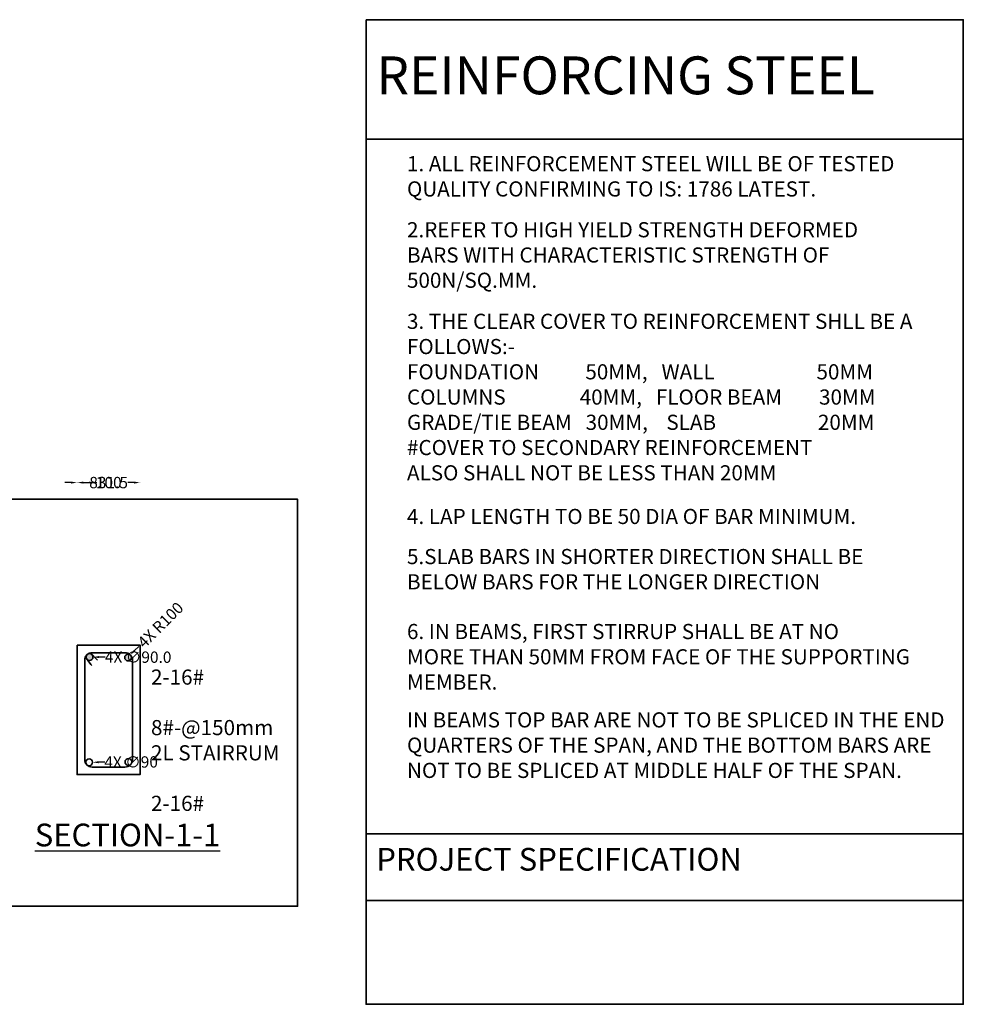
# Model space of a CAD drawing. Units: millimetres. Extents: x -19888 to 14444, y 67066 to 90098.
# Tile 7 of 7: x 1986 to 14444, y 75784 to 88784. Entities that reach past the tile are written whole.
import ezdxf

# ---------------------------------------------------------------- set-up
doc = ezdxf.new("R2010")
doc.units = ezdxf.units.MM
doc.header["$LTSCALE"] = 50
doc.header["$MEASUREMENT"] = 0
for name, color, linetype, lineweight in [('S-ANNO-DIMS', 2, 'Continuous', 18), ('S-ANNO-TEXT', 7, 'Continuous', 25), ('S-ANNO-TTLB', 7, 'Continuous', 35), ('S-BEAM', 3, 'Continuous', 35), ('S-PATT', 8, 'Continuous', 13), ('S-REIN', 6, 'Continuous', 35)]:
    doc.layers.add(name, color=color, linetype=linetype, lineweight=lineweight)
doc.styles.get("Standard").update_dxf_attribs({"font": 'arial.ttf'})
doc.dimstyles.get("Standard").update_dxf_attribs({"dimtxt": 150, "dimasz": 80, "dimexe": 0.18, "dimexo": 0.0625, "dimgap": 0.09, "dimtad": 0, "dimdec": 0, "dimzin": 0, "dimdsep": 46, "dimtxsty": 'Standard', "dimcen": 0.09, "dimadec": 0, "dimazin": 0, "dimtfac": 1, "dimtdec": 0, "dimtofl": 0, "dimtmove": 0, "dimatfit": 3, "dimfxl": 1, "dimfxlon": 1, "dimtolj": 1, "dimtzin": 0, "dimarcsym": 0})

# ---------------------------------------------------------------- blocks, each defined once
blk = doc.blocks.new('*D58')
at = {"layer": 'Defpoints', "color": 0, "ltscale": 50, "transparency": 16777216}
for p in [(3575, 82673), (2744, 80527), (3575, 80527)]:
    blk.add_point(p, dxfattribs=at)
at = {"layer": 'S-ANNO-DIMS', "color": 0, "lineweight": -2, "ltscale": 50, "transparency": 16777216}
for p, q in [((2744, 82672), (2744, 82673)), ((2824, 82673), (2906, 82673)), ((3495, 82673), (3413, 82673)), ((3575, 82672), (3575, 82673))]:
    blk.add_line(p, q, dxfattribs=at)
at = {"layer": 'S-ANNO-DIMS', "color": 0, "ltscale": 50, "transparency": 16777216}
for points in [[(2824, 82686), (2824, 82659), (2744, 82673)], [(3495, 82686), (3495, 82659), (3575, 82673)]]:
    blk.add_solid(points, dxfattribs=at)
at = {"layer": 'S-ANNO-DIMS', "color": 0, "ltscale": 50, "transparency": 16777216, "insert": (3160, 82673), "char_height": 150, "attachment_point": 5}
blk.add_mtext('\\A1;831.5', dxfattribs=at)
blk = doc.blocks.new('*D59')
at = {"layer": 'Defpoints', "color": 0, "ltscale": 50, "transparency": 16777216}
for p in [(2744, 80527), (-9372, 78817), (2744, 78817)]:
    blk.add_point(p, dxfattribs=at)
at = {"layer": 'S-ANNO-DIMS', "color": 0, "lineweight": -2, "ltscale": 50, "transparency": 16777216}
for p, q in [((-9371, 80527), (-9372, 80527)), ((-9372, 80447), (-9372, 79976)), ((-9372, 78897), (-9372, 79367)), ((-9371, 78817), (-9372, 78817))]:
    blk.add_line(p, q, dxfattribs=at)
at = {"layer": 'S-ANNO-DIMS', "color": 0, "ltscale": 50, "transparency": 16777216}
for points in [[(-9385, 80447), (-9359, 80447), (-9372, 80527)], [(-9385, 78897), (-9359, 78897), (-9372, 78817)]]:
    blk.add_solid(points, dxfattribs=at)
at = {"layer": 'S-ANNO-DIMS', "color": 0, "ltscale": 50, "transparency": 16777216, "insert": (-9372, 79672), "char_height": 150, "attachment_point": 5, "rotation": 90}
blk.add_mtext('\\A1;1709.8', dxfattribs=at)
blk = doc.blocks.new('*D60')
at = {"layer": 'Defpoints', "color": 0, "ltscale": 50, "transparency": 16777216}
for p in [(2844, 82673), (2744, 80527), (2844, 80327)]:
    blk.add_point(p, dxfattribs=at)
at = {"layer": 'S-ANNO-DIMS', "color": 0, "lineweight": -2, "ltscale": 50, "transparency": 16777216}
for p, q in [((2664, 82673), (2584, 82673)), ((2744, 82672), (2744, 82673)), ((2844, 82672), (2844, 82673)), ((2924, 82673), (3004, 82673))]:
    blk.add_line(p, q, dxfattribs=at)
at = {"layer": 'S-ANNO-DIMS', "color": 0, "ltscale": 50, "transparency": 16777216}
for points in [[(2664, 82686), (2664, 82659), (2744, 82673)], [(2924, 82686), (2924, 82659), (2844, 82673)]]:
    blk.add_solid(points, dxfattribs=at)
at = {"layer": 'S-ANNO-DIMS', "color": 0, "ltscale": 50, "transparency": 16777216, "insert": (3162, 82673), "char_height": 150, "attachment_point": 5}
blk.add_mtext('\\A1;100', dxfattribs=at)
blk = doc.blocks.new('*D69')
at = {"layer": 'Defpoints', "color": 0, "ltscale": 50, "transparency": 16777216}
for p in [(3446, 80397), (3375, 80327)]:
    blk.add_point(p, dxfattribs=at)
at = {"layer": 'S-ANNO-DIMS', "color": 0, "lineweight": -2, "ltscale": 50, "transparency": 16777216}
for p, q in [((3560, 80510), (3503, 80454)), ((3375, 80327), (3375, 80327)), ((3375, 80327), (3375, 80327))]:
    blk.add_line(p, q, dxfattribs=at)
at = {"layer": 'S-ANNO-DIMS', "color": 0, "ltscale": 50, "transparency": 16777216}
blk.add_solid([(3493, 80463), (3512, 80444), (3446, 80397)], dxfattribs=at)
at = {"layer": 'S-ANNO-DIMS', "color": 0, "ltscale": 50, "transparency": 16777216, "insert": (3844, 80793), "char_height": 150, "attachment_point": 5, "rotation": 44.872}
blk.add_mtext('\\A1;4X R100', dxfattribs=at)
blk = doc.blocks.new('*D70')
at = {"layer": 'Defpoints', "color": 0, "ltscale": 50, "transparency": 16777216}
for p in [(2858, 78979), (2948, 78980)]:
    blk.add_point(p, dxfattribs=at)
at = {"layer": 'S-ANNO-DIMS', "color": 0, "lineweight": -2, "ltscale": 50, "transparency": 16777216}
for p, q in [((2903, 78980), (2903, 78980)), ((2903, 78980), (2903, 78980)), ((3108, 78981), (3028, 78981))]:
    blk.add_line(p, q, dxfattribs=at)
at = {"layer": 'S-ANNO-DIMS', "color": 0, "ltscale": 50, "transparency": 16777216}
blk.add_solid([(3028, 78994), (3028, 78967), (2948, 78980)], dxfattribs=at)
at = {"layer": 'S-ANNO-DIMS', "color": 0, "ltscale": 50, "transparency": 16777216, "insert": (3457, 78983), "char_height": 150, "attachment_point": 5, "rotation": 0.3755}
blk.add_mtext('\\A1;4X ∅90', dxfattribs=at)
blk = doc.blocks.new('*D104')
at = {"layer": 'Defpoints', "color": 0, "ltscale": 50, "transparency": 16777216}
for p in [(2863, 80369), (2953, 80369)]:
    blk.add_point(p, dxfattribs=at)
at = {"layer": 'S-ANNO-DIMS', "color": 0, "lineweight": -2, "ltscale": 50, "transparency": 16777216}
for p, q in [((2908, 80369), (2908, 80369)), ((2908, 80369), (2908, 80369)), ((3113, 80369), (3033, 80369))]:
    blk.add_line(p, q, dxfattribs=at)
at = {"layer": 'S-ANNO-DIMS', "color": 0, "ltscale": 50, "transparency": 16777216}
blk.add_solid([(3033, 80382), (3033, 80355), (2953, 80369)], dxfattribs=at)
at = {"layer": 'S-ANNO-DIMS', "color": 0, "ltscale": 50, "transparency": 16777216, "insert": (3550, 80368), "char_height": 150, "attachment_point": 5, "rotation": 359.8766}
blk.add_mtext('\\A1;4X ∅90.0', dxfattribs=at)

msp = doc.modelspace()

# ---------------------------------------------------------------- hatches: boundary and pattern name
at = {"layer": 'S-PATT', "ltscale": 50}
h = msp.add_hatch(color=256, dxfattribs=at)
h.dxf.hatch_style = 1
h.paths.add_polyline_path([(3375.336, 78916.838, 0.414213562), (3475.336, 79016.838), (3475.336, 80326.651, 0.414213562), (3375.336, 80426.651), (2943.808, 80426.651, 0.414213562), (2843.808, 80326.651), (2843.808, 79016.838, 0.17487802), (2866.844, 78952.991, -0.160250233), (2858.056, 78979.705, -1), (2948.056, 78979.705, -0.647790717), (2873.098, 78946.127, 0.198912367), (2943.808, 78916.838)], flags=0)
h.paths.add_polyline_path([(3446.047, 78946.127, 0.086970776), (3465.88, 78974.39, 0.054595126), (3466.946, 78984.13, 1), (3376.946, 78984.13, 0.591292801)], flags=0)
h.paths.add_polyline_path([(2843.808, 79016.838, 0.414213562), (2943.808, 78916.838), (3375.336, 78916.838, 0.414213562), (3475.336, 79016.838), (3475.336, 80326.651, 0.414213562), (3375.336, 80426.651), (2943.808, 80426.651, 0.15716249), (2885.416, 80407.832, -0.580807732), (2953.319, 80369.096, -1), (2863.319, 80369.096, -0.17989841), (2874.251, 80398.496, 0.203119203), (2843.808, 80326.651)], flags=17)
h.paths.add_polyline_path([(2943.808, 80426.651, 0.414213562), (2843.808, 80326.651), (2843.808, 79016.838, 0.414213562), (2943.808, 78916.838), (3375.336, 78916.838, 0.414213562), (3475.336, 79016.838), (3475.336, 80326.651, 0.159153213), (3456.061, 80385.672, -0.134930588), (3462.383, 80362.672, -1), (3372.383, 80362.672, -0.634413113), (3446.047, 80397.362, 0.198912367), (3375.336, 80426.651)], flags=17)

# ---------------------------------------------------------------- linework, layer by layer
at = {"layer": 'S-ANNO-TTLB', "ltscale": 50}
for p, q in [((6558.599, 87208.092), (14444.195, 87208.092)), ((6558.599, 78036.978), (14444.195, 78036.978)), ((6558.599, 77155.167), (14444.195, 77155.167))]:
    msp.add_line(p, q, dxfattribs=at)
for points in [[(6558.599, 88784.231), (14444.195, 88784.231), (14444.195, 75784.284), (6558.599, 75784.284)], [(-8639.597, 82452.304), (5654.103, 82452.304), (5654.103, 77078.62), (-8639.597, 77078.62)]]:
    msp.add_lwpolyline(points, close=True, dxfattribs=at)
at = {"layer": 'S-BEAM', "ltscale": 50}
msp.add_lwpolyline([(2743.808, 80526.651), (3575.336, 80526.651), (3575.336, 78816.838), (2743.808, 78816.838)], close=True, dxfattribs=at)
at = {"layer": 'S-REIN', "ltscale": 50}
for p, q in [((2852.725, 80367.929), (2925.379, 80272.092)), ((2920.05, 80423.788), (3012.165, 80326.691)), ((2925.379, 80272.092), (2937.608, 80255.961))]:
    msp.add_line(p, q, dxfattribs=at)
msp.add_lwpolyline([(2943.808, 80426.651), (3375.336, 80426.651, -0.414213562), (3475.336, 80326.651), (3475.336, 79016.838, -0.414213562), (3375.336, 78916.838), (2943.808, 78916.838, -0.414213562), (2843.808, 79016.838), (2843.808, 80326.651, -0.414213562)], format="xyb", close=True, dxfattribs=at)
for centre in [(2908.319, 80369.096), (3417.383, 80362.672), (2903.056, 78979.705), (3421.946, 78984.13)]:
    msp.add_circle(centre, 45, dxfattribs=at)

# ---------------------------------------------------------------- texts
at = {"layer": 'S-ANNO-TEXT', "ltscale": 50, "attachment_point": 1}
for s, width, insert, char_height in [('REINFORCING STEEL', 7482.5403, (6693.819, 88299.216), 500), ('1. ALL REINFORCEMENT STEEL WILL BE OF TESTED\\PQUALITY CONFIRMING TO IS: 1786 LATEST.', 7305.15035, (7099.214, 86983.224), 200), ('2.REFER TO HIGH YIELD STRENGTH DEFORMED\\PBARS WITH CHARACTERISTIC STRENGTH OF 500N/SQ.MM.', 7305.15035, (7099.214, 86110.885), 200), ('3. THE CLEAR COVER TO REINFORCEMENT SHLL BE A FOLLOWS:-\\PFOUNDATION          50MM,   WALL                      50MM\\PCOLUMNS                40MM,   FLOOR BEAM        30MM\\PGRADE/TIE BEAM   30MM,    SLAB                      20MM\\P#COVER TO SECONDARY REINFORCEMENT\\PALSO SHALL NOT BE LESS THAN 20MM', 7305.15035, (7099.214, 84902.222), 200), ('4. LAP LENGTH TO BE 50 DIA OF BAR MINIMUM.', 7305.15035, (7099.214, 82325.659), 200), ('5.SLAB BARS IN SHORTER DIRECTION SHALL BE  \\PBELOW BARS FOR THE LONGER DIRECTION', 7305.15035, (7099.214, 81795.932), 200), ('6. IN BEAMS, FIRST STIRRUP SHALL BE AT NO\\PMORE THAN 50MM FROM FACE OF THE SUPPORTING MEMBER.', 7305.15035, (7099.214, 80806.198), 200), ('2-16#\\P\\P8#-@150mm\\P2L STAIRRUM\\P\\P2-16#', 2263.41642, (3719.41, 80204.706), 200), ('IN BEAMS TOP BAR ARE NOT TO BE SPLICED IN THE END QUARTERS OF THE SPAN, AND THE BOTTOM BARS ARE NOT TO BE SPLICED AT MIDDLE HALF OF THE SPAN.', 7305.15035, (7099.214, 79639.462), 200), ('\\pxqc;{\\LSECTION-1-1}', 3602.83103, (1608.529, 78169.735), 300), ('{\\fArial|b1|i0|c0|p34;PROJECT SPECIFICATION}', 8736.78633, (6693.819, 77849.003), 300)]:
    msp.add_mtext_dynamic_manual_height_columns(s, width=width, gutter_width=1, heights=[0], dxfattribs=dict(at, insert=insert, char_height=char_height))

# ---------------------------------------------------------------- dimensions: what is measured, and where the dimension line sits
at = {"layer": 'S-ANNO-DIMS', "ltscale": 50}
for base, p2, override, picture, middle in [((2843.808, 82672.634), (2843.808, 80326.651), {"dimdec": 0, "dimlfac": 1, "dimrnd": 0, "dimzin": 0, "dimdsep": 46, "dimlunit": 2}, '*D60', (3162.289, 82672.634)), ((3575.336, 82672.634), (3575.336, 80526.651), {"dimdec": 1, "dimlfac": 1, "dimrnd": 0, "dimzin": 0, "dimdsep": 46, "dimlunit": 2}, '*D58', (3159.572, 82672.634))]:
    dim = msp.add_linear_dim(base=base, p1=(2743.808, 80526.651), p2=p2, dimstyle='Standard', override=override, dxfattribs=at)
    dim.commit()
    dim.dimension.update_dxf_attribs({"geometry": picture, "text_midpoint": middle})
dim = msp.add_radius_dim(center=(3375.336, 80326.651), mpoint=(3446.205, 80397.204), text='4X <>', dimstyle='Standard', override={"dimdec": 0, "dimlfac": 1, "dimrnd": 0, "dimzin": 0, "dimdsep": 46, "dimlunit": 2}, dxfattribs=at)
dim.commit()
dim.dimension.update_dxf_attribs({"geometry": '*D69', "text_midpoint": (3844.123, 80793.348)})
dim = msp.add_linear_dim(base=(-9372.097, 78816.838), p1=(2743.808, 80526.651), p2=(2743.808, 78816.838), angle=90, dimstyle='Standard', override={"dimdec": 1, "dimlfac": 1, "dimrnd": 0, "dimzin": 0, "dimdsep": 46, "dimlunit": 2}, dxfattribs=at)
dim.commit()
dim.dimension.update_dxf_attribs({"geometry": '*D59', "text_midpoint": (-9372.097, 79671.745)})
dim = msp.add_diameter_dim_2p(p1=(2863.319, 80369.193), p2=(2953.319, 80368.999), text='4X <>', dimstyle='Standard', override={"dimdec": 1, "dimlfac": 1, "dimrnd": 0, "dimzin": 0, "dimdsep": 46, "dimlunit": 2}, dxfattribs=at)
dim.commit()
dim.dimension.update_dxf_attribs({"geometry": '*D104', "text_midpoint": (3549.748, 80367.715), "dimtype": 163})
dim = msp.add_diameter_dim_2p(p1=(2858.057, 78979.411), p2=(2948.055, 78980), text='4X <>', dimstyle='Standard', override={"dimdec": 0, "dimlfac": 1, "dimrnd": 0, "dimzin": 0, "dimdsep": 46, "dimlunit": 2}, dxfattribs=at)
dim.commit()
dim.dimension.update_dxf_attribs({"geometry": '*D70', "text_midpoint": (3457.094, 78983.336)})

doc.saveas('drawing.dxf')
